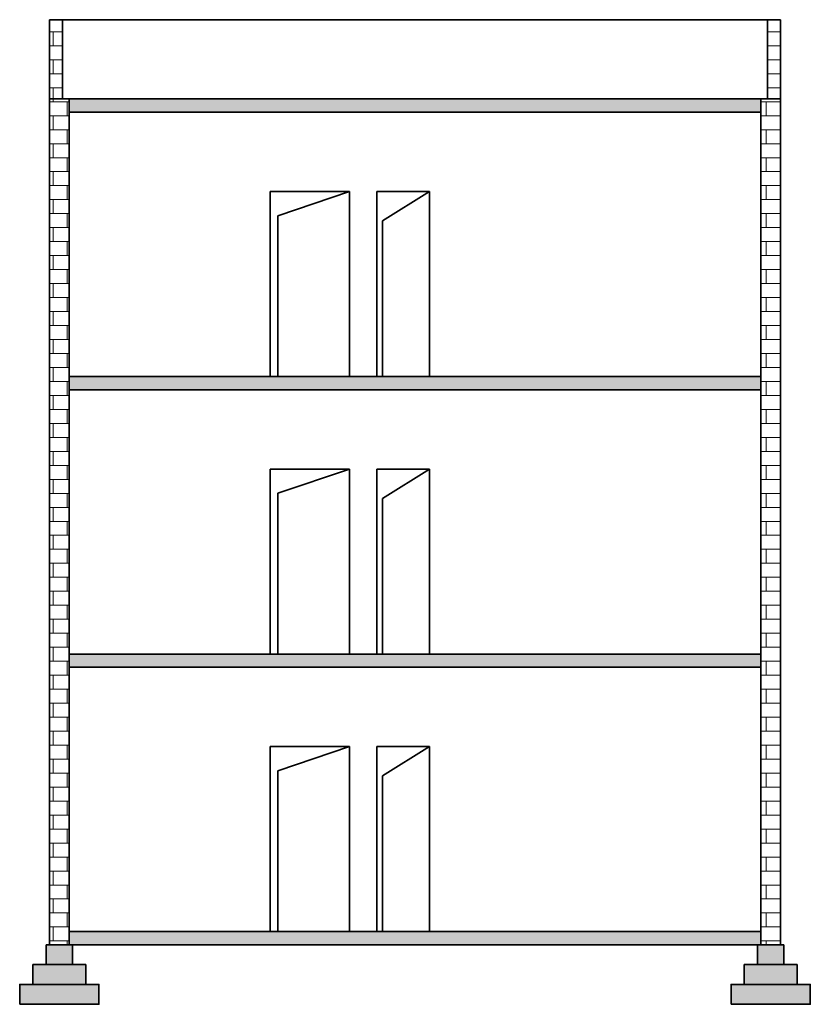
# Model space of a CAD drawing. Units: feet. Extents: x 993 to 3080, y -271 to 22562.
# Tile 3 of 4: x 2436 to 2795, y -271 to 176. Entities that reach past the tile are written whole.
import ezdxf

# ---------------------------------------------------------------- set-up
doc = ezdxf.new("R2010")
doc.units = ezdxf.units.FT
for name, color, linetype, lineweight in [('A-SECT', 7, 'Continuous', 35), ('A-SECT-PATT', 8, 'Continuous', 13), ('S-FNDN', 1, 'Continuous', 35)]:
    doc.layers.add(name, color=color, linetype=linetype, lineweight=lineweight)

# ---------------------------------------------------------------- blocks, each defined once
blk = doc.blocks.new('DOOR-SECT-LEAF-A')
for p, q in [((0, 0), (0, 84)), ((0, 84), (36, 84)), ((3.49, 73.02), (36, 84)), ((36, 84), (36, 0)), ((3.49, 0), (3.49, 73.02))]:
    blk.add_line(p, q)
blk = doc.blocks.new('DOOR-SECT-LEAF-B')
for p, q in [((0, 0), (0, 84)), ((0, 84), (24, 84)), ((2.55, 70.65), (24, 84)), ((24, 84), (24, 0)), ((2.55, 0), (2.55, 70.65))]:
    blk.add_line(p, q)
blk = doc.blocks.new('FOOTING-SECT')
for p, q in [((0, 0), (0, 9)), ((0, 9), (24, 9)), ((24, 9), (24, 0))]:
    blk.add_line(p, q)

msp = doc.modelspace()

# ---------------------------------------------------------------- hatches: boundary and pattern name
at = {"layer": 'A-SECT-PATT'}
h = msp.add_hatch(dxfattribs=at)
h.set_pattern_fill('BRICK', color=256)
h.set_pattern_definition([(0, (1162.2404, 1592.4786), (0, 6.35), []), (90, (1162.24, 1592.479), (-12.7, 8e-16), [6.35, -6.35]), (90, (1168.59, 1592.479), (-12.7, 8e-16), [-6.35, 6.35])])
h.paths.add_polyline_path([(2458.64789, 139.57516), (2449.64789, 139.57516), (2449.64789, 13.57516), (2449.64789, 7.57516), (2449.64789, -112.42484), (2449.64789, -118.42484), (2449.64789, -244.42484), (2458.64789, -244.42484)])
h.paths.add_polyline_path([(2781.64789, 139.57516), (2772.64789, 139.57516), (2772.64789, -244.42484), (2781.64789, -244.42484)])
h.paths.add_polyline_path([(2455.64789, 175.57516), (2449.64789, 175.57516), (2449.64789, 139.57516), (2455.64789, 139.57516)])
h.paths.add_polyline_path([(2781.64789, 175.57516), (2775.64789, 175.57516), (2775.64789, 139.57516), (2781.64789, 139.57516)])
h = msp.add_hatch(dxfattribs=at)
h.set_pattern_fill('AR-SAND', color=256, scale=0.028)
h.set_pattern_definition([(37.5, (1162.2404, 1592.4786), (-0.0448009, 1.37035706), [0, -1.081024, 0, -1.20904, 0, -1.1557]), (7.5, (1162.2404, 1592.4786), (1.2586652, 2.0071103), [0, -0.583184, 0, -0.974344, 0, -0.37338]), (327.5, (1161.3656, 1592.4786), (2.21477864, 0.0040241), [0, -0.3556, 0, -1.28016, 0, -1.67132]), (317.5, (1161.3656, 1592.4786), (2.137958, 0.6242021), [0, -0.1778, 0, -0.839216, 0, -0.96012])])
h.paths.add_polyline_path([(2466.14789, -253.42484), (2442.14789, -253.42484), (2442.14789, -262.42484), (2466.14789, -262.42484)])
h.paths.add_polyline_path([(2789.14789, -253.42484), (2765.14789, -253.42484), (2765.14789, -262.42484), (2789.14789, -262.42484)])
h.paths.add_polyline_path([(2772.64789, -238.42484), (2458.64789, -238.42484), (2458.64789, -244.42484), (2772.64789, -244.42484)])
h.paths.add_polyline_path([(2772.64789, -112.42484), (2458.64789, -112.42484), (2458.64789, -118.42484), (2772.64789, -118.42484)])
h.paths.add_polyline_path([(2772.64789, 139.57516), (2458.64789, 139.57516), (2458.64789, 133.57516), (2772.64789, 133.57516)])
h.paths.add_polyline_path([(2772.64789, 13.57516), (2458.64789, 13.57516), (2458.64789, 7.57516), (2772.64789, 7.57516)])
h = msp.add_hatch(dxfattribs=at)
h.set_pattern_fill('AR-CONC', color=256, scale=0.022)
h.set_pattern_definition([(50, (1162.2404, 1592.4786), (4.0080627, -0.35066), [0.4191, -4.6101]), (355, (1162.2404, 1592.4786), (-0.775355, 4.2032506), [0.33528, -3.688093]), (100.45144, (1162.5744, 1592.4494), (3.2327074, 3.8525905), [0.35618, -3.9179854]), (46.1842, (1162.2404, 1593.596), (5.963739, -0.924931), [0.62865, -6.91515]), (96.63556, (1162.7374, 1593.519), (5.222891, 5.443375), [0.53427, -5.876983]), (351.18415, (1162.2404, 1593.596), (5.222891, 5.443375), [0.50292, -5.532114]), (21, (1162.7992, 1593.3168), (3.3355166, -2.2498344), [0.4191, -4.6101]), (326, (1162.799, 1593.317), (1.3596446, 4.052135), [0.33528, -3.68808]), (71.45144, (1163.077, 1593.1293), (4.695161, 1.802301), [0.35618, -3.9179786]), (37.5, (1162.2404, 1592.4786), (0.0679493, 1.86021086), [0, -3.643376, 0, -3.74396, 0, -3.70205]), (7.5, (1162.2404, 1592.4786), (1.4700326, 2.2039726), [0, -2.134616, 0, -3.559556, 0, -1.41097]), (327.5, (1160.9943, 1592.4786), (2.9829931, -0.1260324), [0, -1.397, 0, -4.35864, 0, -5.78358]), (317.5, (1160.4355, 1592.4786), (3.258842, 0.5593828), [0, -1.8161, 0, -2.894584, 0, -4.10718])])
h.paths.add_polyline_path([(2460.14789, -244.42484), (2449.64789, -244.42484), (2448.14789, -244.42484), (2448.14789, -253.42484), (2460.14789, -253.42484)])
h.paths.add_polyline_path([(2783.14789, -244.42484), (2771.14789, -244.42484), (2771.14789, -253.42484), (2783.14789, -253.42484)])
h = msp.add_hatch(dxfattribs=at)
h.set_pattern_fill('GRAVEL', color=256, scale=0.25)
h.set_pattern_definition([(228.012788, (1166.8124, 1598.8286), (-50.8, -57.15), [0.854304, -84.576209]), (184.969741, (1166.2409, 1598.1936), (76.19999997, 6.350000362), [1.466012, -145.135122]), (132.510447, (1164.7804, 1598.0666), (63.500000027, -69.849999976), [1.033704, -102.336807]), (267.273689, (1162.3039, 1596.4791), (6.350000013, 127), [1.335011, -132.166094]), (292.833654, (1162.2404, 1595.1456), (-31.750000003, 76.2), [1.309084, -129.59952]), (357.273689, (1162.7484, 1593.9391), (-127, 6.350000013), [1.335011, -132.166094]), (37.69424, (1164.0819, 1593.8756), (-82.549999996, -63.500000005), [1.765484, -174.782788]), (72.255328, (1165.4789, 1594.9551), (44.450000012, 139.699999996), [1.666799, -165.013142]), (121.429566, (1165.9869, 1596.5426), (-50.800000007, 82.549999996), [1.339532, -132.613864]), (175.236358, (1165.2884, 1597.6856), (69.85, -6.35000001), [1.529283, -74.934842]), (222.397438, (1163.7644, 1597.8126), (-76.199999998, -69.850000003), [1.977695, -195.791931]), (138.814075, (1168.5904, 1596.4156), (-44.45, 38.1), [0.675011, -66.826415]), (171.469234, (1168.0824, 1596.8601), (82.550000002, -12.699999986), [1.284205, -127.136597]), (225, (1166.8124, 1597.0506), (-9e-16, -6.35), [0.898023, -8.082233]), (203.19859, (1166.3679, 1597.8126), (31.75, 12.7), [0.483603, -47.876556]), (291.80141, (1165.9234, 1597.6221), (-6.35, 19.05), [0.683914, -33.511882]), (30.963757, (1166.1774, 1596.9871), (19.05, 12.7), [1.110799, -35.915745]), (161.56505, (1167.1299, 1597.5586), (12.7, -6.35), [0.803218, -19.277245]), (16.38954, (1162.2404, 1597.6221), (63.5, 19.05), [1.12522, -111.397067]), (70.346176, (1163.3199, 1597.9396), (-25.4, -69.85), [0.943997, -93.455539]), (293.19859, (1167.1299, 1598.8286), (-12.7, 31.75), [0.9672, -47.392959]), (343.61046, (1167.5109, 1597.9396), (-63.5, 19.049999996), [1.12522, -111.397067]), (339.443955, (1162.2404, 1593.6851), (-31.75, 12.7), [1.085088, -53.169336]), (294.77514, (1163.2564, 1593.3041), (-31.75000004, 69.84999998), [0.90918, -90.008983]), (66.80141, (1167.1934, 1592.4786), (12.7, 31.75), [0.9672, -47.392959]), (17.354025, (1167.5744, 1593.3676), (-82.55, -25.400000005), [1.064457, -105.38094]), (69.443955, (1164.0819, 1592.4786), (-12.7, -31.75), [0.542544, -53.71188]), (101.30993, (1166.8124, 1592.4786), (-6.35, 25.4), [0.323786, -32.054987]), (165.96376, (1166.7489, 1592.7961), (19.05, -6.35), [1.309084, -24.872636]), (186.009006, (1165.4789, 1593.1136), (63.5, 6.350000003), [1.213167, -120.103412]), (303.69007, (1166.1774, 1596.4156), (-6.35, 12.7), [0.91581, -21.979441]), (353.157227, (1166.6854, 1595.6536), (107.95, -12.699999994), [1.598892, -158.290023]), (60.945396, (1168.2729, 1595.4631), (-25.4, -44.45), [0.65377, -64.723481]), (90, (1168.5904, 1596.0346), (-6.35, 6.35), [0.381, -5.969]), (120.256437, (1165.3519, 1593.3041), (25.4, -44.45), [0.882167, -87.334852]), (48.012787, (1164.9074, 1594.0661), (50.8, 57.15), [1.708607, -83.721905]), (0, (1166.0504, 1595.336), (6.35, 6.35), [1.651, -4.699]), (325.304846, (1167.7014, 1595.3361), (63.500000024, -44.449999966), [1.004024, -99.398292]), (254.054604, (1168.5269, 1594.7646), (-6.35, -25.4), [0.924573, -45.304125]), (207.645975, (1168.2729, 1593.8756), (-120.650000004, -63.499999992), [1.505363, -149.031161]), (175.426079, (1166.9394, 1593.1771), (-82.55, 6.35), [1.592574, -157.664616])])
h.paths.add_polyline_path([(2472.14789, -262.42484), (2436.14789, -262.42484), (2436.14789, -271.42484), (2472.14789, -271.42484)])
h.paths.add_polyline_path([(2795.14789, -262.42484), (2759.14789, -262.42484), (2759.14789, -271.42484), (2795.14789, -271.42484)])

# ---------------------------------------------------------------- linework, layer by layer
at = {"layer": 'A-SECT'}
for p, q in [((2449.64789, 13.57516), (2449.64789, 175.57516)), ((2449.64789, 175.57516), (2781.64789, 175.57516)), ((2449.64789, 175.57516), (2449.64789, 175.57516)), ((2455.64789, 175.57516), (2455.64789, 139.57516)), ((2775.64789, 175.57516), (2775.64789, 139.57516)), ((2781.64789, -244.42484), (2781.64789, 175.57516)), ((2449.64789, 139.57516), (2781.64789, 139.57516)), ((2458.64789, 139.57516), (2458.64789, -244.42484)), ((2772.64789, 139.57516), (2772.64789, -244.42484)), ((2458.64789, 133.57516), (2772.64789, 133.57516)), ((2449.64789, 7.57516), (2449.64789, 13.57516)), ((2458.64789, 13.57516), (2772.64789, 13.57516)), ((2449.64789, -112.42484), (2449.64789, 7.57516)), ((2458.64789, 7.57516), (2772.64789, 7.57516)), ((2449.64789, -118.42484), (2449.64789, -112.42484)), ((2458.64789, -112.42484), (2772.64789, -112.42484)), ((2449.64789, -244.42484), (2449.64789, -118.42484)), ((2458.64789, -118.42484), (2772.64789, -118.42484)), ((2458.64789, -238.42484), (2772.64789, -238.42484)), ((2448.14789, -253.42484), (2448.14789, -244.42484)), ((2448.14789, -244.42484), (2460.14789, -244.42484)), ((2449.64789, -244.42484), (2781.64789, -244.42484)), ((2449.64789, -244.42484), (2458.64789, -244.42484)), ((2460.14789, -244.42484), (2460.14789, -253.42484)), ((2771.14789, -253.42484), (2771.14789, -244.42484)), ((2771.14789, -244.42484), (2783.14789, -244.42484)), ((2772.64789, -244.42484), (2781.64789, -244.42484)), ((2783.14789, -244.42484), (2783.14789, -253.42484))]:
    msp.add_line(p, q, dxfattribs=at)
for points in [[(2436.14789, -271.42484), (2472.14789, -271.42484), (2472.14789, -262.42484), (2436.14789, -262.42484)], [(2759.14789, -271.42484), (2795.14789, -271.42484), (2795.14789, -262.42484), (2759.14789, -262.42484)]]:
    msp.add_lwpolyline(points, close=True, dxfattribs=at)

# ---------------------------------------------------------------- block references
for name, p in [('DOOR-SECT-LEAF-A', (2549.924, 13.575)), ('DOOR-SECT-LEAF-B', (2598.3, 13.575)), ('DOOR-SECT-LEAF-A', (2549.924, -112.425)), ('DOOR-SECT-LEAF-B', (2598.3, -112.425)), ('DOOR-SECT-LEAF-A', (2549.924, -238.425)), ('DOOR-SECT-LEAF-B', (2598.3, -238.425))]:
    msp.add_blockref(name, p, dxfattribs=at)
at = {"layer": 'S-FNDN'}
for p in [(2442.148, -262.425), (2765.148, -262.425)]:
    msp.add_blockref('FOOTING-SECT', p, dxfattribs=at)

doc.saveas('drawing.dxf')
